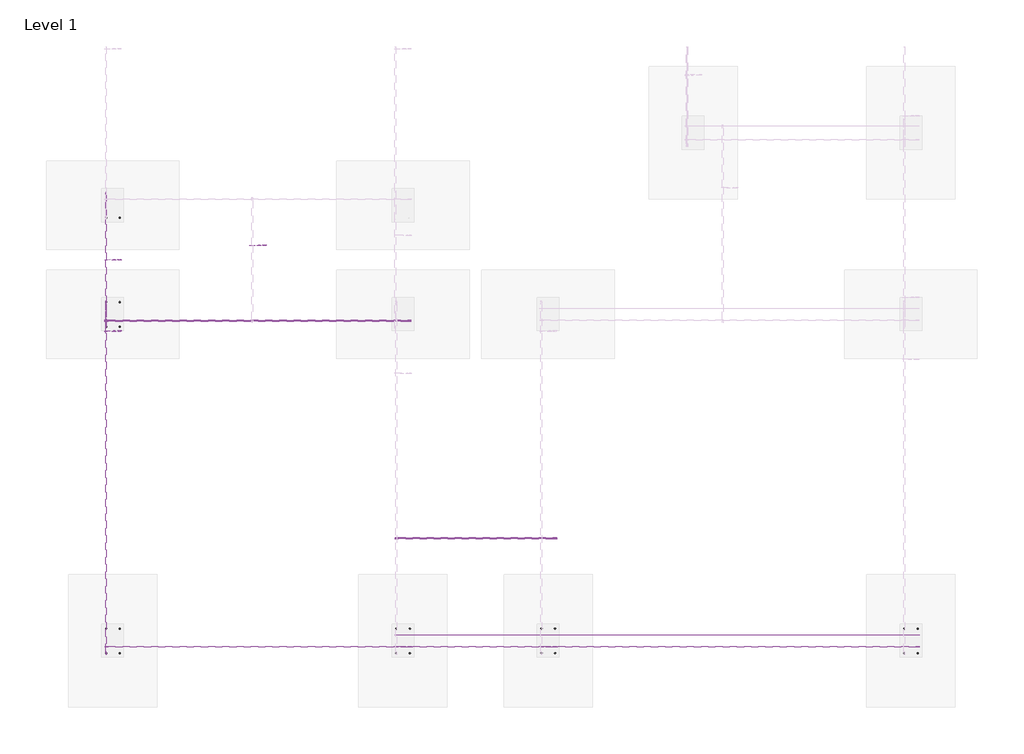
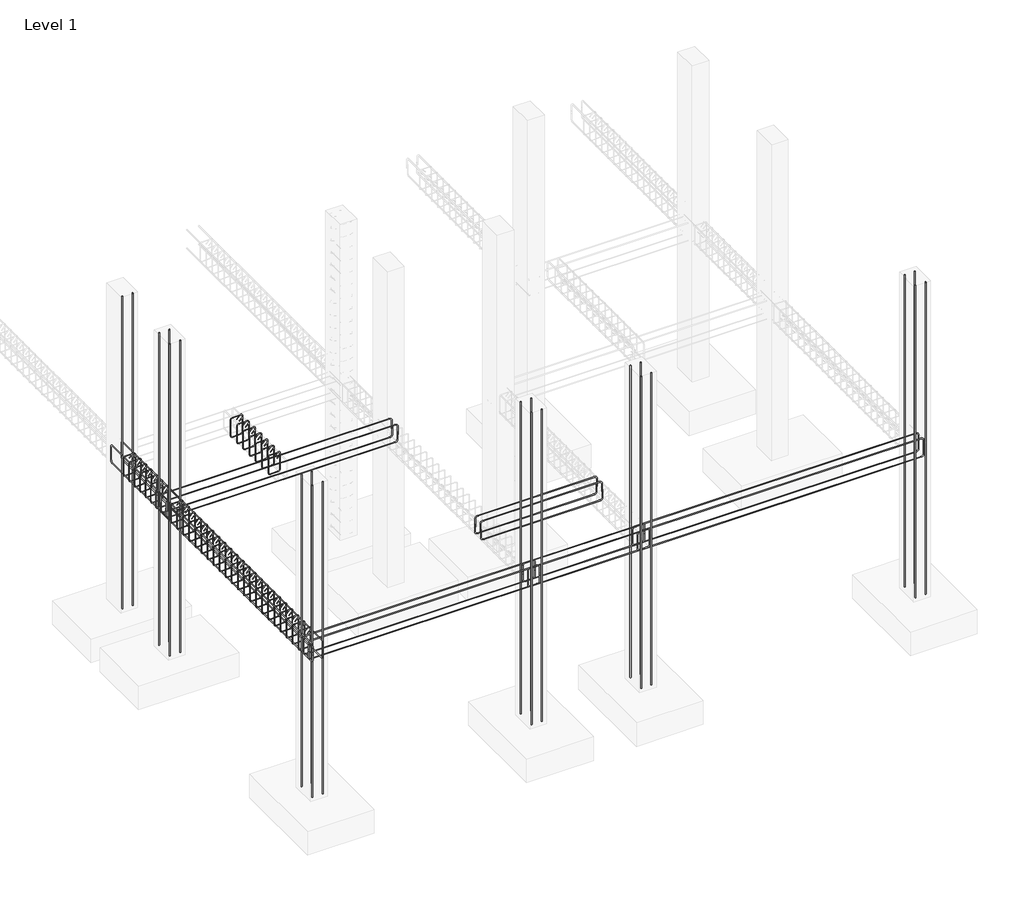
# One storey, part 2 of 5: 28 reinforcing bars.
"""IFC4 building model written with IfcOpenShell, lengths in millimetres."""

from ifc_helpers import new_model, si_unit, point, frame, origin, place, context, project, spatial, polyline, circle_curve, trimmed, segment, composite_curve, source, transform, mapped, element, save
from ifc_brep_helpers import swept_disk

model = new_model("IFC4")

# Units and contexts
model_context = context("Model", 3, world=origin())
ifc_project = project(units=[si_unit("LENGTHUNIT", "METRE", prefix="MILLI")], contexts=[model_context])

# Site, building, storey
site = spatial("IfcSite", under=ifc_project)
building = spatial("IfcBuilding", under=site)
storey = spatial("IfcBuildingStorey", under=building, Name="Level 1", Elevation=0.0)

# Reinforcing bars
placement = place(None, origin())
reinforcing_bar_shape = source(origin(), model_context, "Body", "SolidModel", [
    swept_disk(composite_curve([segment(polyline([(-4213.892587, -1952.6442969, 38.1), (-4213.892587, -1952.6442969, 6057.9)]), True, "CONTINUOUS")], self_intersect=False), 8.001),
])
element("IfcReinforcingBar", 1, at=placement, inside=storey, context=model_context, shape_type="MappedRepresentation", body=[
    mapped(reinforcing_bar_shape, transform((0.0, 0.0, 0.0), x_axis=(1.0, 0.0, 0.0), y_axis=(0.0, 1.0, 0.0), z_axis=(0.0, 0.0, 1.0))),
    mapped(reinforcing_bar_shape, transform((-186.6579018, 0.0, 0.0), x_axis=(1.0, 0.0, 0.0), y_axis=(0.0, 1.0, 0.0), z_axis=(0.0, 0.0, 1.0))),
])
reinforcing_bar_2_shape = source(origin(), model_context, "Body", "SolidModel", [
    swept_disk(composite_curve([segment(polyline([(-4213.892587, -2291.7021987, 6057.9), (-4213.892587, -2291.7021987, 38.1)]), True, "CONTINUOUS")], self_intersect=False), 8.001),
])
element("IfcReinforcingBar", 2, at=placement, inside=storey, context=model_context, shape_type="MappedRepresentation", body=[
    mapped(reinforcing_bar_2_shape, transform((0.0, 0.0, 0.0), x_axis=(1.0, 0.0, 0.0), y_axis=(0.0, 1.0, 0.0), z_axis=(0.0, 0.0, 1.0))),
    mapped(reinforcing_bar_2_shape, transform((-186.6579018, 0.0, 0.0), x_axis=(1.0, 0.0, 0.0), y_axis=(0.0, 1.0, 0.0), z_axis=(0.0, 0.0, 1.0))),
])
reinforcing_bar_3_shape = source(origin(), model_context, "Body", "SolidModel", [
    swept_disk(composite_curve([segment(polyline([(-15212.455746, 4062.3577522, 2793.8967919), (-15212.455746, 4062.3577522, 2946.2967919)]), True, "CONTINUOUS"), segment(trimmed(circle_curve(frame((-15212.455746, 4018.2887522, 2946.2967919), z_axis=(1.0, 0.0, 0.0), x_axis=(0.0, 44.06899999999996, 0.0)), 44.069), [point((-15212.455746, 4062.3577522, 2946.2967919))], [point((-15212.455746, 4018.2887522, 2990.3657919))], True, "CARTESIAN"), True, "CONTINUOUS"), segment(polyline([(-15212.455746, 4018.2887522, 2990.3657919), (-15212.455746, 2237.3647522, 2990.3657919)]), True, "CONTINUOUS"), segment(trimmed(circle_curve(frame((-15212.455746, 2237.3647522, 2946.2967919), z_axis=(1.0, 0.0, 0.0), x_axis=(0.0, 0.0, 44.069000000000415)), 44.069), [point((-15212.455746, 2237.3647522, 2990.3657919))], [point((-15212.455746, 2193.2957522, 2946.2967919))], True, "CARTESIAN"), True, "CONTINUOUS"), segment(polyline([(-15212.455746, 2193.2957522, 2946.2967919), (-15212.455746, 2193.2957522, 2793.8967919)]), True, "CONTINUOUS")], self_intersect=False), 5.969),
])
element("IfcReinforcingBar", 3, at=placement, inside=storey, context=model_context, shape_type="MappedRepresentation", body=[
    mapped(reinforcing_bar_3_shape, transform((0.0, 0.0, 0.0), x_axis=(1.0, 0.0, 0.0), y_axis=(0.0, 1.0, 0.0), z_axis=(0.0, 0.0, 1.0))),
    mapped(reinforcing_bar_3_shape, transform((-189.5315837, 0.0, 0.0), x_axis=(1.0, 0.0, 0.0), y_axis=(0.0, 1.0, 0.0), z_axis=(0.0, 0.0, 1.0))),
])
reinforcing_bar_4_shape = source(origin(), model_context, "Body", "SolidModel", [
    swept_disk(composite_curve([segment(polyline([(-15212.455746, 2193.2957522, 2844.9032081), (-15212.455746, 2193.2957522, 2692.5032081)]), True, "CONTINUOUS"), segment(trimmed(circle_curve(frame((-15212.455746, 2237.3647522, 2692.5032081), z_axis=(1.0, 0.0, 0.0), x_axis=(0.0, -44.06899999999996, 0.0)), 44.069), [point((-15212.455746, 2193.2957522, 2692.5032081))], [point((-15212.455746, 2237.3647522, 2648.4342081))], True, "CARTESIAN"), True, "CONTINUOUS"), segment(polyline([(-15212.455746, 2237.3647522, 2648.4342081), (-15212.455746, 4018.2887522, 2648.4342081)]), True, "CONTINUOUS"), segment(trimmed(circle_curve(frame((-15212.455746, 4018.2887522, 2692.5032081), z_axis=(1.0, 0.0, 0.0), x_axis=(0.0, 0.0, -44.06899999999996)), 44.069), [point((-15212.455746, 4018.2887522, 2648.4342081))], [point((-15212.455746, 4062.3577522, 2692.5032081))], True, "CARTESIAN"), True, "CONTINUOUS"), segment(polyline([(-15212.455746, 4062.3577522, 2692.5032081), (-15212.455746, 4062.3577522, 2844.9032081)]), True, "CONTINUOUS")], self_intersect=False), 5.969),
])
element("IfcReinforcingBar", 4, at=placement, inside=storey, context=model_context, shape_type="MappedRepresentation", body=[
    mapped(reinforcing_bar_4_shape, transform((0.0, 0.0, 0.0), x_axis=(1.0, 0.0, 0.0), y_axis=(0.0, 1.0, 0.0), z_axis=(0.0, 0.0, 1.0))),
    mapped(reinforcing_bar_4_shape, transform((-189.5315837, 0.0, 0.0), x_axis=(1.0, 0.0, 0.0), y_axis=(0.0, 1.0, 0.0), z_axis=(0.0, 0.0, 1.0))),
])
reinforcing_bar_5_shape = source(origin(), model_context, "Body", "SolidModel", [
    swept_disk(composite_curve([segment(polyline([(-15212.455746, 2562.3577522, 2793.8967919), (-15212.455746, 2562.3577522, 2946.2967919)]), True, "CONTINUOUS"), segment(trimmed(circle_curve(frame((-15212.455746, 2518.2887522, 2946.2967919), z_axis=(1.0, 0.0, 0.0), x_axis=(0.0, 44.06899999999996, 0.0)), 44.069), [point((-15212.455746, 2562.3577522, 2946.2967919))], [point((-15212.455746, 2518.2887522, 2990.3657919))], True, "CARTESIAN"), True, "CONTINUOUS"), segment(polyline([(-15212.455746, 2518.2887522, 2990.3657919), (-15212.455746, -2262.6352478, 2990.3657919)]), True, "CONTINUOUS"), segment(trimmed(circle_curve(frame((-15212.455746, -2262.6352478, 2946.2967919), z_axis=(1.0, 0.0, 0.0), x_axis=(0.0, 0.0, 44.069000000000415)), 44.069), [point((-15212.455746, -2262.6352478, 2990.3657919))], [point((-15212.455746, -2306.7042478, 2946.2967919))], True, "CARTESIAN"), True, "CONTINUOUS"), segment(polyline([(-15212.455746, -2306.7042478, 2946.2967919), (-15212.455746, -2306.7042478, 2793.8967919)]), True, "CONTINUOUS")], self_intersect=False), 5.969),
])
element("IfcReinforcingBar", 5, at=placement, inside=storey, context=model_context, shape_type="MappedRepresentation", body=[
    mapped(reinforcing_bar_5_shape, transform((0.0, 0.0, 0.0), x_axis=(1.0, 0.0, 0.0), y_axis=(0.0, 1.0, 0.0), z_axis=(0.0, 0.0, 1.0))),
    mapped(reinforcing_bar_5_shape, transform((-189.5315837, 0.0, 0.0), x_axis=(1.0, 0.0, 0.0), y_axis=(0.0, 1.0, 0.0), z_axis=(0.0, 0.0, 1.0))),
])
reinforcing_bar_6_shape = source(origin(), model_context, "Body", "SolidModel", [
    swept_disk(composite_curve([segment(polyline([(-15212.455746, -2306.7042478, 2844.9032081), (-15212.455746, -2306.7042478, 2692.5032081)]), True, "CONTINUOUS"), segment(trimmed(circle_curve(frame((-15212.455746, -2262.6352478, 2692.5032081), z_axis=(1.0, 0.0, 0.0), x_axis=(0.0, -44.06899999999996, 0.0)), 44.069), [point((-15212.455746, -2306.7042478, 2692.5032081))], [point((-15212.455746, -2262.6352478, 2648.4342081))], True, "CARTESIAN"), True, "CONTINUOUS"), segment(polyline([(-15212.455746, -2262.6352478, 2648.4342081), (-15212.455746, 2518.2887522, 2648.4342081)]), True, "CONTINUOUS"), segment(trimmed(circle_curve(frame((-15212.455746, 2518.2887522, 2692.5032081), z_axis=(1.0, 0.0, 0.0), x_axis=(0.0, 0.0, -44.06899999999996)), 44.069), [point((-15212.455746, 2518.2887522, 2648.4342081))], [point((-15212.455746, 2562.3577522, 2692.5032081))], True, "CARTESIAN"), True, "CONTINUOUS"), segment(polyline([(-15212.455746, 2562.3577522, 2692.5032081), (-15212.455746, 2562.3577522, 2844.9032081)]), True, "CONTINUOUS")], self_intersect=False), 5.969),
])
element("IfcReinforcingBar", 6, at=placement, inside=storey, context=model_context, shape_type="MappedRepresentation", body=[
    mapped(reinforcing_bar_6_shape, transform((0.0, 0.0, 0.0), x_axis=(1.0, 0.0, 0.0), y_axis=(0.0, 1.0, 0.0), z_axis=(0.0, 0.0, 1.0))),
    mapped(reinforcing_bar_6_shape, transform((-189.5315837, 0.0, 0.0), x_axis=(1.0, 0.0, 0.0), y_axis=(0.0, 1.0, 0.0), z_axis=(0.0, 0.0, 1.0))),
])
reinforcing_bar_7_shape = source(origin(), model_context, "Body", "SolidModel", [
    swept_disk(composite_curve([segment(polyline([(-15213.892587, 3708.2978013, 6057.9), (-15213.892587, 3708.2978013, 38.1)]), True, "CONTINUOUS")], self_intersect=False), 8.001),
])
element("IfcReinforcingBar", 7, at=placement, inside=storey, context=model_context, shape_type="MappedRepresentation", body=[
    mapped(reinforcing_bar_7_shape, transform((0.0, 0.0, 0.0), x_axis=(1.0, 0.0, 0.0), y_axis=(0.0, 1.0, 0.0), z_axis=(0.0, 0.0, 1.0))),
    mapped(reinforcing_bar_7_shape, transform((-186.6579018, 0.0, 0.0), x_axis=(1.0, 0.0, 0.0), y_axis=(0.0, 1.0, 0.0), z_axis=(0.0, 0.0, 1.0))),
])
reinforcing_bar_8_shape = source(origin(), model_context, "Body", "SolidModel", [
    swept_disk(composite_curve([segment(polyline([(-15213.892587, 2547.3557031, 38.1), (-15213.892587, 2547.3557031, 6057.9)]), True, "CONTINUOUS")], self_intersect=False), 8.001),
])
element("IfcReinforcingBar", 8, at=placement, inside=storey, context=model_context, shape_type="MappedRepresentation", body=[
    mapped(reinforcing_bar_8_shape, transform((0.0, 0.0, 0.0), x_axis=(1.0, 0.0, 0.0), y_axis=(0.0, 1.0, 0.0), z_axis=(0.0, 0.0, 1.0))),
    mapped(reinforcing_bar_8_shape, transform((-186.6579018, 0.0, 0.0), x_axis=(1.0, 0.0, 0.0), y_axis=(0.0, 1.0, 0.0), z_axis=(0.0, 0.0, 1.0))),
])
reinforcing_bar_9_shape = source(origin(), model_context, "Body", "SolidModel", [
    swept_disk(composite_curve([segment(polyline([(-15213.892587, 2208.2978013, 6057.9), (-15213.892587, 2208.2978013, 38.1)]), True, "CONTINUOUS")], self_intersect=False), 8.001),
])
element("IfcReinforcingBar", 9, at=placement, inside=storey, context=model_context, shape_type="MappedRepresentation", body=[
    mapped(reinforcing_bar_9_shape, transform((0.0, 0.0, 0.0), x_axis=(1.0, 0.0, 0.0), y_axis=(0.0, 1.0, 0.0), z_axis=(0.0, 0.0, 1.0))),
    mapped(reinforcing_bar_9_shape, transform((-186.6579018, 0.0, 0.0), x_axis=(1.0, 0.0, 0.0), y_axis=(0.0, 1.0, 0.0), z_axis=(0.0, 0.0, 1.0))),
])
reinforcing_bar_10_shape = source(origin(), model_context, "Body", "SolidModel", [
    swept_disk(composite_curve([segment(polyline([(-15213.892587, -1952.6442969, 38.1), (-15213.892587, -1952.6442969, 6057.9)]), True, "CONTINUOUS")], self_intersect=False), 8.001),
])
element("IfcReinforcingBar", 10, at=placement, inside=storey, context=model_context, shape_type="MappedRepresentation", body=[
    mapped(reinforcing_bar_10_shape, transform((0.0, 0.0, 0.0), x_axis=(1.0, 0.0, 0.0), y_axis=(0.0, 1.0, 0.0), z_axis=(0.0, 0.0, 1.0))),
    mapped(reinforcing_bar_10_shape, transform((-186.6579018, 0.0, 0.0), x_axis=(1.0, 0.0, 0.0), y_axis=(0.0, 1.0, 0.0), z_axis=(0.0, 0.0, 1.0))),
])
reinforcing_bar_11_shape = source(origin(), model_context, "Body", "SolidModel", [
    swept_disk(composite_curve([segment(polyline([(-15213.892587, -2291.7021987, 6057.9), (-15213.892587, -2291.7021987, 38.1)]), True, "CONTINUOUS")], self_intersect=False), 8.001),
])
element("IfcReinforcingBar", 11, at=placement, inside=storey, context=model_context, shape_type="MappedRepresentation", body=[
    mapped(reinforcing_bar_11_shape, transform((0.0, 0.0, 0.0), x_axis=(1.0, 0.0, 0.0), y_axis=(0.0, 1.0, 0.0), z_axis=(0.0, 0.0, 1.0))),
    mapped(reinforcing_bar_11_shape, transform((-186.6579018, 0.0, 0.0), x_axis=(1.0, 0.0, 0.0), y_axis=(0.0, 1.0, 0.0), z_axis=(0.0, 0.0, 1.0))),
])
reinforcing_bar_12_shape = source(origin(), model_context, "Body", "SolidModel", [
    swept_disk(composite_curve([segment(polyline([(-15260.3161447, 3645.2897522, 2901.0166099), (-15205.4511463, 3645.2897522, 2955.8816084)]), True, "CONTINUOUS"), segment(trimmed(circle_curve(frame((-15226.1955379, 3645.2897522, 2976.626), z_axis=(0.0, -1.0, 0.0), x_axis=(20.74439159999929, 0.0, -20.7443916000002)), 29.337), [point((-15205.4511463, 3645.2897522, 2955.8816084))], [point((-15226.1955379, 3645.2897522, 3005.963))], True, "CARTESIAN"), True, "CONTINUOUS"), segment(polyline([(-15226.1955379, 3645.2897522, 3005.963), (-15388.2475379, 3645.2897522, 3005.963)]), True, "CONTINUOUS"), segment(trimmed(circle_curve(frame((-15388.2475379, 3645.2897522, 2976.626), z_axis=(0.0, -1.0, 0.0), x_axis=(0.0, 0.0, 29.33699999999999)), 29.337), [point((-15388.2475379, 3645.2897522, 3005.963))], [point((-15417.5845379, 3645.2897522, 2976.626))], True, "CARTESIAN"), True, "CONTINUOUS"), segment(polyline([(-15417.5845379, 3645.2897522, 2976.626), (-15417.5845379, 3645.2897522, 2662.174)]), True, "CONTINUOUS"), segment(trimmed(circle_curve(frame((-15388.2661869, 3646.3356312, 2662.174), z_axis=(0.03565051078635061, -0.9993643184948482, 0.0), x_axis=(-29.318350999999893, -1.045879000000241, 0.0)), 29.337), [point((-15417.5845379, 3645.2897522, 2662.174))], [point((-15388.2661869, 3646.3356312, 2632.837))], True, "CARTESIAN"), True, "CONTINUOUS"), segment(polyline([(-15388.2661869, 3646.3356312, 2632.837), (-15226.1768889, 3652.1178731, 2632.837)]), True, "CONTINUOUS"), segment(trimmed(circle_curve(frame((-15226.1768889, 3652.1178731, 2662.174), z_axis=(0.03565051078635061, -0.9993643184948482, 0.0), x_axis=(0.0, 0.0, -29.33699999999999)), 29.337), [point((-15226.1768889, 3652.1178731, 2632.837))], [point((-15196.8585379, 3653.1637522, 2662.174))], True, "CARTESIAN"), True, "CONTINUOUS"), segment(polyline([(-15196.8585379, 3653.1637522, 2662.174), (-15196.8585379, 3653.1637522, 2976.626)]), True, "CONTINUOUS"), segment(trimmed(circle_curve(frame((-15226.1955379, 3653.1637522, 2976.626), z_axis=(0.0, -1.0, 0.0), x_axis=(29.336999999999534, 0.0, 0.0)), 29.337), [point((-15196.8585379, 3653.1637522, 2976.626))], [point((-15246.9399295, 3653.1637522, 2997.3703916))], True, "CARTESIAN"), True, "CONTINUOUS"), segment(polyline([(-15246.9399295, 3653.1637522, 2997.3703916), (-15301.804928, 3653.1637522, 2942.5053932)]), True, "CONTINUOUS")], self_intersect=False), 3.937),
])
element("IfcReinforcingBar", 12, at=placement, inside=storey, context=model_context, shape_type="MappedRepresentation", body=[
    mapped(reinforcing_bar_12_shape, transform((0.0, 0.0, 0.0), x_axis=(1.0, 0.0, 0.0), y_axis=(0.0, 1.0, 0.0), z_axis=(0.0, 0.0, 1.0))),
    mapped(reinforcing_bar_12_shape, transform((0.0, -172.4876667, 0.0), x_axis=(1.0, 0.0, 0.0), y_axis=(0.0, 1.0, 0.0), z_axis=(0.0, 0.0, 1.0))),
    mapped(reinforcing_bar_12_shape, transform((0.0, -344.9753333, 0.0), x_axis=(1.0, 0.0, 0.0), y_axis=(0.0, 1.0, 0.0), z_axis=(0.0, 0.0, 1.0))),
    mapped(reinforcing_bar_12_shape, transform((0.0, -517.463, 0.0), x_axis=(1.0, 0.0, 0.0), y_axis=(0.0, 1.0, 0.0), z_axis=(0.0, 0.0, 1.0))),
    mapped(reinforcing_bar_12_shape, transform((0.0, -689.9506667, 0.0), x_axis=(1.0, 0.0, 0.0), y_axis=(0.0, 1.0, 0.0), z_axis=(0.0, 0.0, 1.0))),
    mapped(reinforcing_bar_12_shape, transform((0.0, -862.4383333, 0.0), x_axis=(1.0, 0.0, 0.0), y_axis=(0.0, 1.0, 0.0), z_axis=(0.0, 0.0, 1.0))),
    mapped(reinforcing_bar_12_shape, transform((0.0, -1034.926, 0.0), x_axis=(1.0, 0.0, 0.0), y_axis=(0.0, 1.0, 0.0), z_axis=(0.0, 0.0, 1.0))),
])
reinforcing_bar_13_shape = source(origin(), model_context, "Body", "SolidModel", [
    swept_disk(composite_curve([segment(polyline([(-15260.3161447, 2145.2897522, 2901.0166099), (-15205.4511463, 2145.2897522, 2955.8816084)]), True, "CONTINUOUS"), segment(trimmed(circle_curve(frame((-15226.1955379, 2145.2897522, 2976.626), z_axis=(0.0, -1.0, 0.0), x_axis=(20.74439159999929, 0.0, -20.7443916000002)), 29.337), [point((-15205.4511463, 2145.2897522, 2955.8816084))], [point((-15226.1955379, 2145.2897522, 3005.963))], True, "CARTESIAN"), True, "CONTINUOUS"), segment(polyline([(-15226.1955379, 2145.2897522, 3005.963), (-15388.2475379, 2145.2897522, 3005.963)]), True, "CONTINUOUS"), segment(trimmed(circle_curve(frame((-15388.2475379, 2145.2897522, 2976.626), z_axis=(0.0, -1.0, 0.0), x_axis=(0.0, 0.0, 29.33699999999999)), 29.337), [point((-15388.2475379, 2145.2897522, 3005.963))], [point((-15417.5845379, 2145.2897522, 2976.626))], True, "CARTESIAN"), True, "CONTINUOUS"), segment(polyline([(-15417.5845379, 2145.2897522, 2976.626), (-15417.5845379, 2145.2897522, 2662.174)]), True, "CONTINUOUS"), segment(trimmed(circle_curve(frame((-15388.2661869, 2146.3356312, 2662.174), z_axis=(0.03565051078634999, -0.9993643184948483, 0.0), x_axis=(-29.318350999999893, -1.045879000000241, 0.0)), 29.337), [point((-15417.5845379, 2145.2897522, 2662.174))], [point((-15388.2661869, 2146.3356312, 2632.837))], True, "CARTESIAN"), True, "CONTINUOUS"), segment(polyline([(-15388.2661869, 2146.3356312, 2632.837), (-15226.1768889, 2152.1178731, 2632.837)]), True, "CONTINUOUS"), segment(trimmed(circle_curve(frame((-15226.1768889, 2152.1178731, 2662.174), z_axis=(0.03565051078634999, -0.9993643184948483, 0.0), x_axis=(0.0, 0.0, -29.33699999999999)), 29.337), [point((-15226.1768889, 2152.1178731, 2632.837))], [point((-15196.8585379, 2153.1637522, 2662.174))], True, "CARTESIAN"), True, "CONTINUOUS"), segment(polyline([(-15196.8585379, 2153.1637522, 2662.174), (-15196.8585379, 2153.1637522, 2976.626)]), True, "CONTINUOUS"), segment(trimmed(circle_curve(frame((-15226.1955379, 2153.1637522, 2976.626), z_axis=(0.0, -1.0, 0.0), x_axis=(29.336999999999534, 0.0, 0.0)), 29.337), [point((-15196.8585379, 2153.1637522, 2976.626))], [point((-15246.9399295, 2153.1637522, 2997.3703916))], True, "CARTESIAN"), True, "CONTINUOUS"), segment(polyline([(-15246.9399295, 2153.1637522, 2997.3703916), (-15301.804928, 2153.1637522, 2942.5053932)]), True, "CONTINUOUS")], self_intersect=False), 3.937),
])
element("IfcReinforcingBar", 13, at=placement, inside=storey, context=model_context, shape_type="MappedRepresentation", body=[
    mapped(reinforcing_bar_13_shape, transform((0.0, 0.0, 0.0), x_axis=(1.0, 0.0, 0.0), y_axis=(0.0, 1.0, 0.0), z_axis=(0.0, 0.0, 1.0))),
    mapped(reinforcing_bar_13_shape, transform((0.0, -192.1393333, 0.0), x_axis=(1.0, 0.0, 0.0), y_axis=(0.0, 1.0, 0.0), z_axis=(0.0, 0.0, 1.0))),
    mapped(reinforcing_bar_13_shape, transform((0.0, -384.2786667, 0.0), x_axis=(1.0, 0.0, 0.0), y_axis=(0.0, 1.0, 0.0), z_axis=(0.0, 0.0, 1.0))),
    mapped(reinforcing_bar_13_shape, transform((0.0, -576.418, 0.0), x_axis=(1.0, 0.0, 0.0), y_axis=(0.0, 1.0, 0.0), z_axis=(0.0, 0.0, 1.0))),
    mapped(reinforcing_bar_13_shape, transform((0.0, -768.5573333, 0.0), x_axis=(1.0, 0.0, 0.0), y_axis=(0.0, 1.0, 0.0), z_axis=(0.0, 0.0, 1.0))),
    mapped(reinforcing_bar_13_shape, transform((0.0, -960.6966667, 0.0), x_axis=(1.0, 0.0, 0.0), y_axis=(0.0, 1.0, 0.0), z_axis=(0.0, 0.0, 1.0))),
    mapped(reinforcing_bar_13_shape, transform((0.0, -1152.836, 0.0), x_axis=(1.0, 0.0, 0.0), y_axis=(0.0, 1.0, 0.0), z_axis=(0.0, 0.0, 1.0))),
    mapped(reinforcing_bar_13_shape, transform((0.0, -1344.9753333, 0.0), x_axis=(1.0, 0.0, 0.0), y_axis=(0.0, 1.0, 0.0), z_axis=(0.0, 0.0, 1.0))),
    mapped(reinforcing_bar_13_shape, transform((0.0, -1537.1146667, 0.0), x_axis=(1.0, 0.0, 0.0), y_axis=(0.0, 1.0, 0.0), z_axis=(0.0, 0.0, 1.0))),
    mapped(reinforcing_bar_13_shape, transform((0.0, -1729.254, 0.0), x_axis=(1.0, 0.0, 0.0), y_axis=(0.0, 1.0, 0.0), z_axis=(0.0, 0.0, 1.0))),
    mapped(reinforcing_bar_13_shape, transform((0.0, -1921.3933333, 0.0), x_axis=(1.0, 0.0, 0.0), y_axis=(0.0, 1.0, 0.0), z_axis=(0.0, 0.0, 1.0))),
    mapped(reinforcing_bar_13_shape, transform((0.0, -2113.5326667, 0.0), x_axis=(1.0, 0.0, 0.0), y_axis=(0.0, 1.0, 0.0), z_axis=(0.0, 0.0, 1.0))),
    mapped(reinforcing_bar_13_shape, transform((0.0, -2305.672, 0.0), x_axis=(1.0, 0.0, 0.0), y_axis=(0.0, 1.0, 0.0), z_axis=(0.0, 0.0, 1.0))),
    mapped(reinforcing_bar_13_shape, transform((0.0, -2497.8113333, 0.0), x_axis=(1.0, 0.0, 0.0), y_axis=(0.0, 1.0, 0.0), z_axis=(0.0, 0.0, 1.0))),
    mapped(reinforcing_bar_13_shape, transform((0.0, -2689.9506667, 0.0), x_axis=(1.0, 0.0, 0.0), y_axis=(0.0, 1.0, 0.0), z_axis=(0.0, 0.0, 1.0))),
    mapped(reinforcing_bar_13_shape, transform((0.0, -2882.09, 0.0), x_axis=(1.0, 0.0, 0.0), y_axis=(0.0, 1.0, 0.0), z_axis=(0.0, 0.0, 1.0))),
    mapped(reinforcing_bar_13_shape, transform((0.0, -3074.2293333, 0.0), x_axis=(1.0, 0.0, 0.0), y_axis=(0.0, 1.0, 0.0), z_axis=(0.0, 0.0, 1.0))),
    mapped(reinforcing_bar_13_shape, transform((0.0, -3266.3686667, 0.0), x_axis=(1.0, 0.0, 0.0), y_axis=(0.0, 1.0, 0.0), z_axis=(0.0, 0.0, 1.0))),
    mapped(reinforcing_bar_13_shape, transform((0.0, -3458.508, 0.0), x_axis=(1.0, 0.0, 0.0), y_axis=(0.0, 1.0, 0.0), z_axis=(0.0, 0.0, 1.0))),
    mapped(reinforcing_bar_13_shape, transform((0.0, -3650.6473333, 0.0), x_axis=(1.0, 0.0, 0.0), y_axis=(0.0, 1.0, 0.0), z_axis=(0.0, 0.0, 1.0))),
    mapped(reinforcing_bar_13_shape, transform((0.0, -3842.7866667, 0.0), x_axis=(1.0, 0.0, 0.0), y_axis=(0.0, 1.0, 0.0), z_axis=(0.0, 0.0, 1.0))),
    mapped(reinforcing_bar_13_shape, transform((0.0, -4034.926, 0.0), x_axis=(1.0, 0.0, 0.0), y_axis=(0.0, 1.0, 0.0), z_axis=(0.0, 0.0, 1.0))),
])
reinforcing_bar_14_shape = source(origin(), model_context, "Body", "SolidModel", [
    swept_disk(composite_curve([segment(polyline([(-13260.3161447, 3721.4897522, 2901.0166099), (-13205.4511463, 3721.4897522, 2955.8816084)]), True, "CONTINUOUS"), segment(trimmed(circle_curve(frame((-13226.1955379, 3721.4897522, 2976.626), z_axis=(0.0, -1.0, 0.0), x_axis=(20.74439159999929, 0.0, -20.7443916000002)), 29.337), [point((-13205.4511463, 3721.4897522, 2955.8816084))], [point((-13226.1955379, 3721.4897522, 3005.963))], True, "CARTESIAN"), True, "CONTINUOUS"), segment(polyline([(-13226.1955379, 3721.4897522, 3005.963), (-13388.2475379, 3721.4897522, 3005.963)]), True, "CONTINUOUS"), segment(trimmed(circle_curve(frame((-13388.2475379, 3721.4897522, 2976.626), z_axis=(0.0, -1.0, 0.0), x_axis=(0.0, 0.0, 29.33699999999999)), 29.337), [point((-13388.2475379, 3721.4897522, 3005.963))], [point((-13417.5845379, 3721.4897522, 2976.626))], True, "CARTESIAN"), True, "CONTINUOUS"), segment(polyline([(-13417.5845379, 3721.4897522, 2976.626), (-13417.5845379, 3721.4897522, 2662.174)]), True, "CONTINUOUS"), segment(trimmed(circle_curve(frame((-13388.2661869, 3722.5356312, 2662.174), z_axis=(0.035650510786350516, -0.9993643184948482, 0.0), x_axis=(-29.318350999999893, -1.0458789999997862, 0.0)), 29.337), [point((-13417.5845379, 3721.4897522, 2662.174))], [point((-13388.2661869, 3722.5356312, 2632.837))], True, "CARTESIAN"), True, "CONTINUOUS"), segment(polyline([(-13388.2661869, 3722.5356312, 2632.837), (-13226.1768889, 3728.3178731, 2632.837)]), True, "CONTINUOUS"), segment(trimmed(circle_curve(frame((-13226.1768889, 3728.3178731, 2662.174), z_axis=(0.035650510786350516, -0.9993643184948482, 0.0), x_axis=(0.0, 0.0, -29.33699999999999)), 29.337), [point((-13226.1768889, 3728.3178731, 2632.837))], [point((-13196.8585379, 3729.3637522, 2662.174))], True, "CARTESIAN"), True, "CONTINUOUS"), segment(polyline([(-13196.8585379, 3729.3637522, 2662.174), (-13196.8585379, 3729.3637522, 2976.626)]), True, "CONTINUOUS"), segment(trimmed(circle_curve(frame((-13226.1955379, 3729.3637522, 2976.626), z_axis=(0.0, -1.0, 0.0), x_axis=(29.336999999999534, 0.0, 0.0)), 29.337), [point((-13196.8585379, 3729.3637522, 2976.626))], [point((-13246.9399295, 3729.3637522, 2997.3703916))], True, "CARTESIAN"), True, "CONTINUOUS"), segment(polyline([(-13246.9399295, 3729.3637522, 2997.3703916), (-13301.804928, 3729.3637522, 2942.5053932)]), True, "CONTINUOUS")], self_intersect=False), 3.937),
])
element("IfcReinforcingBar", 14, at=placement, inside=storey, context=model_context, shape_type="MappedRepresentation", body=[
    mapped(reinforcing_bar_14_shape, transform((0.0, 0.0, 0.0), x_axis=(1.0, 0.0, 0.0), y_axis=(0.0, 1.0, 0.0), z_axis=(0.0, 0.0, 1.0))),
    mapped(reinforcing_bar_14_shape, transform((0.0, -197.8876667, 0.0), x_axis=(1.0, 0.0, 0.0), y_axis=(0.0, 1.0, 0.0), z_axis=(0.0, 0.0, 1.0))),
    mapped(reinforcing_bar_14_shape, transform((0.0, -395.7753333, 0.0), x_axis=(1.0, 0.0, 0.0), y_axis=(0.0, 1.0, 0.0), z_axis=(0.0, 0.0, 1.0))),
    mapped(reinforcing_bar_14_shape, transform((0.0, -593.663, 0.0), x_axis=(1.0, 0.0, 0.0), y_axis=(0.0, 1.0, 0.0), z_axis=(0.0, 0.0, 1.0))),
    mapped(reinforcing_bar_14_shape, transform((0.0, -791.5506667, 0.0), x_axis=(1.0, 0.0, 0.0), y_axis=(0.0, 1.0, 0.0), z_axis=(0.0, 0.0, 1.0))),
    mapped(reinforcing_bar_14_shape, transform((0.0, -989.4383333, 0.0), x_axis=(1.0, 0.0, 0.0), y_axis=(0.0, 1.0, 0.0), z_axis=(0.0, 0.0, 1.0))),
    mapped(reinforcing_bar_14_shape, transform((0.0, -1187.326, 0.0), x_axis=(1.0, 0.0, 0.0), y_axis=(0.0, 1.0, 0.0), z_axis=(0.0, 0.0, 1.0))),
])
reinforcing_bar_15_shape = source(origin(), model_context, "Body", "SolidModel", [
    swept_disk(composite_curve([segment(polyline([(-11198.8905379, 2283.0609603, 2793.8967919), (-11198.8905379, 2283.0609603, 2946.2967919)]), True, "CONTINUOUS"), segment(trimmed(circle_curve(frame((-11242.9595379, 2283.0609603, 2946.2967919), z_axis=(0.0, -1.0, 0.0), x_axis=(44.068999999999505, 0.0, 0.0)), 44.069), [point((-11198.8905379, 2283.0609603, 2946.2967919))], [point((-11242.9595379, 2283.0609603, 2990.3657919))], True, "CARTESIAN"), True, "CONTINUOUS"), segment(polyline([(-11242.9595379, 2283.0609603, 2990.3657919), (-15371.4835379, 2283.0609603, 2990.3657919)]), True, "CONTINUOUS"), segment(trimmed(circle_curve(frame((-15371.4835379, 2283.0609603, 2946.2967919), z_axis=(0.0, -1.0, 0.0), x_axis=(0.0, 0.0, 44.069000000000415)), 44.069), [point((-15371.4835379, 2283.0609603, 2990.3657919))], [point((-15415.5525379, 2283.0609603, 2946.2967919))], True, "CARTESIAN"), True, "CONTINUOUS"), segment(polyline([(-15415.5525379, 2283.0609603, 2946.2967919), (-15415.5525379, 2283.0609603, 2793.8967919)]), True, "CONTINUOUS")], self_intersect=False), 5.969),
])
element("IfcReinforcingBar", 15, at=placement, inside=storey, context=model_context, shape_type="MappedRepresentation", body=[
    mapped(reinforcing_bar_15_shape, transform((0.0, 0.0, 0.0), x_axis=(1.0, 0.0, 0.0), y_axis=(0.0, 1.0, 0.0), z_axis=(0.0, 0.0, 1.0))),
    mapped(reinforcing_bar_15_shape, transform((0.0, 189.5315837, 0.0), x_axis=(1.0, 0.0, 0.0), y_axis=(0.0, 1.0, 0.0), z_axis=(0.0, 0.0, 1.0))),
])
reinforcing_bar_16_shape = source(origin(), model_context, "Body", "SolidModel", [
    swept_disk(composite_curve([segment(polyline([(-15415.5525379, 2458.8527522, 2839.212), (-15415.5525379, 2458.8527522, 2686.812)]), True, "CONTINUOUS"), segment(trimmed(circle_curve(frame((-15371.4835379, 2458.8527522, 2686.812), z_axis=(0.0, -1.0, 0.0), x_axis=(-44.068999999999505, 0.0, 0.0)), 44.069), [point((-15415.5525379, 2458.8527522, 2686.812))], [point((-15371.4835379, 2458.8527522, 2642.743))], True, "CARTESIAN"), True, "CONTINUOUS"), segment(polyline([(-15371.4835379, 2458.8527522, 2642.743), (-11242.9595379, 2458.8527522, 2642.743)]), True, "CONTINUOUS"), segment(trimmed(circle_curve(frame((-11242.9595379, 2458.8527522, 2686.812), z_axis=(0.0, -1.0, 0.0), x_axis=(0.0, 0.0, -44.06899999999996)), 44.069), [point((-11242.9595379, 2458.8527522, 2642.743))], [point((-11198.8905379, 2458.8527522, 2686.812))], True, "CARTESIAN"), True, "CONTINUOUS"), segment(polyline([(-11198.8905379, 2458.8527522, 2686.812), (-11198.8905379, 2458.8527522, 2839.212)]), True, "CONTINUOUS")], self_intersect=False), 5.969),
])
element("IfcReinforcingBar", 16, at=placement, inside=storey, context=model_context, shape_type="MappedRepresentation", body=[
    mapped(reinforcing_bar_16_shape, transform((0.0, 0.0, 0.0), x_axis=(1.0, 0.0, 0.0), y_axis=(0.0, 1.0, 0.0), z_axis=(0.0, 0.0, 1.0))),
    mapped(reinforcing_bar_16_shape, transform((0.0, -162.052, 0.0), x_axis=(1.0, 0.0, 0.0), y_axis=(0.0, 1.0, 0.0), z_axis=(0.0, 0.0, 1.0))),
])
reinforcing_bar_17_shape = source(origin(), model_context, "Body", "SolidModel", [
    swept_disk(composite_curve([segment(polyline([(-11213.892587, -1952.6442969, 38.1), (-11213.892587, -1952.6442969, 6057.9)]), True, "CONTINUOUS")], self_intersect=False), 8.001),
])
element("IfcReinforcingBar", 17, at=placement, inside=storey, context=model_context, shape_type="MappedRepresentation", body=[
    mapped(reinforcing_bar_17_shape, transform((0.0, 0.0, 0.0), x_axis=(1.0, 0.0, 0.0), y_axis=(0.0, 1.0, 0.0), z_axis=(0.0, 0.0, 1.0))),
    mapped(reinforcing_bar_17_shape, transform((-186.6579018, 0.0, 0.0), x_axis=(1.0, 0.0, 0.0), y_axis=(0.0, 1.0, 0.0), z_axis=(0.0, 0.0, 1.0))),
])
reinforcing_bar_18_shape = source(origin(), model_context, "Body", "SolidModel", [
    swept_disk(composite_curve([segment(polyline([(-11213.892587, -2291.7021987, 6057.9), (-11213.892587, -2291.7021987, 38.1)]), True, "CONTINUOUS")], self_intersect=False), 8.001),
])
element("IfcReinforcingBar", 18, at=placement, inside=storey, context=model_context, shape_type="MappedRepresentation", body=[
    mapped(reinforcing_bar_18_shape, transform((0.0, 0.0, 0.0), x_axis=(1.0, 0.0, 0.0), y_axis=(0.0, 1.0, 0.0), z_axis=(0.0, 0.0, 1.0))),
    mapped(reinforcing_bar_18_shape, transform((-186.6579018, 0.0, 0.0), x_axis=(1.0, 0.0, 0.0), y_axis=(0.0, 1.0, 0.0), z_axis=(0.0, 0.0, 1.0))),
])
reinforcing_bar_19_shape = source(origin(), model_context, "Body", "SolidModel", [
    swept_disk(composite_curve([segment(polyline([(-9198.8905379, -541.1472478, 2799.588), (-9198.8905379, -541.1472478, 2951.988)]), True, "CONTINUOUS"), segment(trimmed(circle_curve(frame((-9242.9595379, -541.1472478, 2951.988), z_axis=(0.0, -1.0, 0.0), x_axis=(44.068999999999505, 0.0, 0.0)), 44.069), [point((-9198.8905379, -541.1472478, 2951.988))], [point((-9242.9595379, -541.1472478, 2996.057))], True, "CARTESIAN"), True, "CONTINUOUS"), segment(polyline([(-9242.9595379, -541.1472478, 2996.057), (-11371.4835379, -541.1472478, 2996.057)]), True, "CONTINUOUS"), segment(trimmed(circle_curve(frame((-11371.4835379, -541.1472478, 2951.988), z_axis=(0.0, -1.0, 0.0), x_axis=(0.0, 0.0, 44.06899999999996)), 44.069), [point((-11371.4835379, -541.1472478, 2996.057))], [point((-11415.5525379, -541.1472478, 2951.988))], True, "CARTESIAN"), True, "CONTINUOUS"), segment(polyline([(-11415.5525379, -541.1472478, 2951.988), (-11415.5525379, -541.1472478, 2799.588)]), True, "CONTINUOUS")], self_intersect=False), 5.969),
])
element("IfcReinforcingBar", 19, at=placement, inside=storey, context=model_context, shape_type="MappedRepresentation", body=[
    mapped(reinforcing_bar_19_shape, transform((0.0, 0.0, 0.0), x_axis=(1.0, 0.0, 0.0), y_axis=(0.0, 1.0, 0.0), z_axis=(0.0, 0.0, 1.0))),
    mapped(reinforcing_bar_19_shape, transform((0.0, -162.052, 0.0), x_axis=(1.0, 0.0, 0.0), y_axis=(0.0, 1.0, 0.0), z_axis=(0.0, 0.0, 1.0))),
])
reinforcing_bar_20_shape = source(origin(), model_context, "Body", "SolidModel", [
    swept_disk(composite_curve([segment(polyline([(-11415.5525379, -716.9390397, 2844.9032081), (-11415.5525379, -716.9390397, 2692.5032081)]), True, "CONTINUOUS"), segment(trimmed(circle_curve(frame((-11371.4835379, -716.9390397, 2692.5032081), z_axis=(0.0, -1.0, 0.0), x_axis=(-44.068999999999505, 0.0, 0.0)), 44.069), [point((-11415.5525379, -716.9390397, 2692.5032081))], [point((-11371.4835379, -716.9390397, 2648.4342081))], True, "CARTESIAN"), True, "CONTINUOUS"), segment(polyline([(-11371.4835379, -716.9390397, 2648.4342081), (-9242.9595379, -716.9390397, 2648.4342081)]), True, "CONTINUOUS"), segment(trimmed(circle_curve(frame((-9242.9595379, -716.9390397, 2692.5032081), z_axis=(0.0, -1.0, 0.0), x_axis=(0.0, 0.0, -44.06899999999996)), 44.069), [point((-9242.9595379, -716.9390397, 2648.4342081))], [point((-9198.8905379, -716.9390397, 2692.5032081))], True, "CARTESIAN"), True, "CONTINUOUS"), segment(polyline([(-9198.8905379, -716.9390397, 2692.5032081), (-9198.8905379, -716.9390397, 2844.9032081)]), True, "CONTINUOUS")], self_intersect=False), 5.969),
])
element("IfcReinforcingBar", 20, at=placement, inside=storey, context=model_context, shape_type="MappedRepresentation", body=[
    mapped(reinforcing_bar_20_shape, transform((0.0, 0.0, 0.0), x_axis=(1.0, 0.0, 0.0), y_axis=(0.0, 1.0, 0.0), z_axis=(0.0, 0.0, 1.0))),
    mapped(reinforcing_bar_20_shape, transform((0.0, 189.5315837, 0.0), x_axis=(1.0, 0.0, 0.0), y_axis=(0.0, 1.0, 0.0), z_axis=(0.0, 0.0, 1.0))),
])
reinforcing_bar_21_shape = source(origin(), model_context, "Body", "SolidModel", [
    swept_disk(composite_curve([segment(polyline([(-9213.892587, -2291.7021987, 6057.9), (-9213.892587, -2291.7021987, 38.1)]), True, "CONTINUOUS")], self_intersect=False), 8.001),
])
element("IfcReinforcingBar", 21, at=placement, inside=storey, context=model_context, shape_type="MappedRepresentation", body=[
    mapped(reinforcing_bar_21_shape, transform((0.0, 0.0, 0.0), x_axis=(1.0, 0.0, 0.0), y_axis=(0.0, 1.0, 0.0), z_axis=(0.0, 0.0, 1.0))),
    mapped(reinforcing_bar_21_shape, transform((-186.6579018, 0.0, 0.0), x_axis=(1.0, 0.0, 0.0), y_axis=(0.0, 1.0, 0.0), z_axis=(0.0, 0.0, 1.0))),
])
reinforcing_bar_22_shape = source(origin(), model_context, "Body", "SolidModel", [
    swept_disk(composite_curve([segment(polyline([(-9213.892587, -1952.6442969, 38.1), (-9213.892587, -1952.6442969, 6057.9)]), True, "CONTINUOUS")], self_intersect=False), 8.001),
])
element("IfcReinforcingBar", 22, at=placement, inside=storey, context=model_context, shape_type="MappedRepresentation", body=[
    mapped(reinforcing_bar_22_shape, transform((0.0, 0.0, 0.0), x_axis=(1.0, 0.0, 0.0), y_axis=(0.0, 1.0, 0.0), z_axis=(0.0, 0.0, 1.0))),
    mapped(reinforcing_bar_22_shape, transform((-186.6579018, 0.0, 0.0), x_axis=(1.0, 0.0, 0.0), y_axis=(0.0, 1.0, 0.0), z_axis=(0.0, 0.0, 1.0))),
])
reinforcing_bar_23_shape = source(origin(), model_context, "Body", "SolidModel", [
    swept_disk(composite_curve([segment(polyline([(-4198.8905379, -2041.1472478, 2799.588), (-4198.8905379, -2041.1472478, 2951.988)]), True, "CONTINUOUS"), segment(trimmed(circle_curve(frame((-4242.9595379, -2041.1472478, 2951.988), z_axis=(0.0, -1.0, 0.0), x_axis=(44.069000000000415, 0.0, 0.0)), 44.069), [point((-4198.8905379, -2041.1472478, 2951.988))], [point((-4242.9595379, -2041.1472478, 2996.057))], True, "CARTESIAN"), True, "CONTINUOUS"), segment(polyline([(-4242.9595379, -2041.1472478, 2996.057), (-9371.4835379, -2041.1472478, 2996.057)]), True, "CONTINUOUS"), segment(trimmed(circle_curve(frame((-9371.4835379, -2041.1472478, 2951.988), z_axis=(0.0, -1.0, 0.0), x_axis=(0.0, 0.0, 44.06899999999996)), 44.069), [point((-9371.4835379, -2041.1472478, 2996.057))], [point((-9415.5525379, -2041.1472478, 2951.988))], True, "CARTESIAN"), True, "CONTINUOUS"), segment(polyline([(-9415.5525379, -2041.1472478, 2951.988), (-9415.5525379, -2041.1472478, 2799.588)]), True, "CONTINUOUS")], self_intersect=False), 5.969),
])
element("IfcReinforcingBar", 23, at=placement, inside=storey, context=model_context, shape_type="MappedRepresentation", body=[
    mapped(reinforcing_bar_23_shape, transform((0.0, 0.0, 0.0), x_axis=(1.0, 0.0, 0.0), y_axis=(0.0, 1.0, 0.0), z_axis=(0.0, 0.0, 1.0))),
    mapped(reinforcing_bar_23_shape, transform((0.0, -162.052, 0.0), x_axis=(1.0, 0.0, 0.0), y_axis=(0.0, 1.0, 0.0), z_axis=(0.0, 0.0, 1.0))),
])
reinforcing_bar_24_shape = source(origin(), model_context, "Body", "SolidModel", [
    swept_disk(composite_curve([segment(polyline([(-9415.5525379, -2203.1992478, 2839.212), (-9415.5525379, -2203.1992478, 2686.812)]), True, "CONTINUOUS"), segment(trimmed(circle_curve(frame((-9371.4835379, -2203.1992478, 2686.812), z_axis=(0.0, -1.0, 0.0), x_axis=(-44.068999999999505, 0.0, 0.0)), 44.069), [point((-9415.5525379, -2203.1992478, 2686.812))], [point((-9371.4835379, -2203.1992478, 2642.743))], True, "CARTESIAN"), True, "CONTINUOUS"), segment(polyline([(-9371.4835379, -2203.1992478, 2642.743), (-4242.9595379, -2203.1992478, 2642.743)]), True, "CONTINUOUS"), segment(trimmed(circle_curve(frame((-4242.9595379, -2203.1992478, 2686.812), z_axis=(0.0, -1.0, 0.0), x_axis=(0.0, 0.0, -44.06899999999996)), 44.069), [point((-4242.9595379, -2203.1992478, 2642.743))], [point((-4198.8905379, -2203.1992478, 2686.812))], True, "CARTESIAN"), True, "CONTINUOUS"), segment(polyline([(-4198.8905379, -2203.1992478, 2686.812), (-4198.8905379, -2203.1992478, 2839.212)]), True, "CONTINUOUS")], self_intersect=False), 5.969),
])
element("IfcReinforcingBar", 24, at=placement, inside=storey, context=model_context, shape_type="MappedRepresentation", body=[
    mapped(reinforcing_bar_24_shape, transform((0.0, 0.0, 0.0), x_axis=(1.0, 0.0, 0.0), y_axis=(0.0, 1.0, 0.0), z_axis=(0.0, 0.0, 1.0))),
    mapped(reinforcing_bar_24_shape, transform((0.0, 162.052, 0.0), x_axis=(1.0, 0.0, 0.0), y_axis=(0.0, 1.0, 0.0), z_axis=(0.0, 0.0, 1.0))),
])
reinforcing_bar_25_shape = source(origin(), model_context, "Body", "SolidModel", [
    swept_disk(composite_curve([segment(polyline([(-9198.8905379, -2041.1472478, 2799.588), (-9198.8905379, -2041.1472478, 2951.988)]), True, "CONTINUOUS"), segment(trimmed(circle_curve(frame((-9242.9595379, -2041.1472478, 2951.988), z_axis=(0.0, -1.0, 0.0), x_axis=(44.068999999999505, 0.0, 0.0)), 44.069), [point((-9198.8905379, -2041.1472478, 2951.988))], [point((-9242.9595379, -2041.1472478, 2996.057))], True, "CARTESIAN"), True, "CONTINUOUS"), segment(polyline([(-9242.9595379, -2041.1472478, 2996.057), (-11371.4835379, -2041.1472478, 2996.057)]), True, "CONTINUOUS"), segment(trimmed(circle_curve(frame((-11371.4835379, -2041.1472478, 2951.988), z_axis=(0.0, -1.0, 0.0), x_axis=(0.0, 0.0, 44.06899999999996)), 44.069), [point((-11371.4835379, -2041.1472478, 2996.057))], [point((-11415.5525379, -2041.1472478, 2951.988))], True, "CARTESIAN"), True, "CONTINUOUS"), segment(polyline([(-11415.5525379, -2041.1472478, 2951.988), (-11415.5525379, -2041.1472478, 2799.588)]), True, "CONTINUOUS")], self_intersect=False), 5.969),
])
element("IfcReinforcingBar", 25, at=placement, inside=storey, context=model_context, shape_type="MappedRepresentation", body=[
    mapped(reinforcing_bar_25_shape, transform((0.0, 0.0, 0.0), x_axis=(1.0, 0.0, 0.0), y_axis=(0.0, 1.0, 0.0), z_axis=(0.0, 0.0, 1.0))),
    mapped(reinforcing_bar_25_shape, transform((0.0, -162.052, 0.0), x_axis=(1.0, 0.0, 0.0), y_axis=(0.0, 1.0, 0.0), z_axis=(0.0, 0.0, 1.0))),
])
reinforcing_bar_26_shape = source(origin(), model_context, "Body", "SolidModel", [
    swept_disk(composite_curve([segment(polyline([(-11415.5525379, -2203.1992478, 2839.212), (-11415.5525379, -2203.1992478, 2686.812)]), True, "CONTINUOUS"), segment(trimmed(circle_curve(frame((-11371.4835379, -2203.1992478, 2686.812), z_axis=(0.0, -1.0, 0.0), x_axis=(-44.068999999999505, 0.0, 0.0)), 44.069), [point((-11415.5525379, -2203.1992478, 2686.812))], [point((-11371.4835379, -2203.1992478, 2642.743))], True, "CARTESIAN"), True, "CONTINUOUS"), segment(polyline([(-11371.4835379, -2203.1992478, 2642.743), (-9242.9595379, -2203.1992478, 2642.743)]), True, "CONTINUOUS"), segment(trimmed(circle_curve(frame((-9242.9595379, -2203.1992478, 2686.812), z_axis=(0.0, -1.0, 0.0), x_axis=(0.0, 0.0, -44.06899999999996)), 44.069), [point((-9242.9595379, -2203.1992478, 2642.743))], [point((-9198.8905379, -2203.1992478, 2686.812))], True, "CARTESIAN"), True, "CONTINUOUS"), segment(polyline([(-9198.8905379, -2203.1992478, 2686.812), (-9198.8905379, -2203.1992478, 2839.212)]), True, "CONTINUOUS")], self_intersect=False), 5.969),
])
element("IfcReinforcingBar", 26, at=placement, inside=storey, context=model_context, shape_type="MappedRepresentation", body=[
    mapped(reinforcing_bar_26_shape, transform((0.0, 0.0, 0.0), x_axis=(1.0, 0.0, 0.0), y_axis=(0.0, 1.0, 0.0), z_axis=(0.0, 0.0, 1.0))),
    mapped(reinforcing_bar_26_shape, transform((0.0, 162.052, 0.0), x_axis=(1.0, 0.0, 0.0), y_axis=(0.0, 1.0, 0.0), z_axis=(0.0, 0.0, 1.0))),
])
reinforcing_bar_27_shape = source(origin(), model_context, "Body", "SolidModel", [
    swept_disk(composite_curve([segment(polyline([(-11198.8905379, -2041.1472478, 2799.588), (-11198.8905379, -2041.1472478, 2951.988)]), True, "CONTINUOUS"), segment(trimmed(circle_curve(frame((-11242.9595379, -2041.1472478, 2951.988), z_axis=(0.0, -1.0, 0.0), x_axis=(44.068999999999505, 0.0, 0.0)), 44.069), [point((-11198.8905379, -2041.1472478, 2951.988))], [point((-11242.9595379, -2041.1472478, 2996.057))], True, "CARTESIAN"), True, "CONTINUOUS"), segment(polyline([(-11242.9595379, -2041.1472478, 2996.057), (-15371.4835379, -2041.1472478, 2996.057)]), True, "CONTINUOUS"), segment(trimmed(circle_curve(frame((-15371.4835379, -2041.1472478, 2951.988), z_axis=(0.0, -1.0, 0.0), x_axis=(0.0, 0.0, 44.06899999999996)), 44.069), [point((-15371.4835379, -2041.1472478, 2996.057))], [point((-15415.5525379, -2041.1472478, 2951.988))], True, "CARTESIAN"), True, "CONTINUOUS"), segment(polyline([(-15415.5525379, -2041.1472478, 2951.988), (-15415.5525379, -2041.1472478, 2799.588)]), True, "CONTINUOUS")], self_intersect=False), 5.969),
])
element("IfcReinforcingBar", 27, at=placement, inside=storey, context=model_context, shape_type="MappedRepresentation", body=[
    mapped(reinforcing_bar_27_shape, transform((0.0, 0.0, 0.0), x_axis=(1.0, 0.0, 0.0), y_axis=(0.0, 1.0, 0.0), z_axis=(0.0, 0.0, 1.0))),
    mapped(reinforcing_bar_27_shape, transform((0.0, -162.052, 0.0), x_axis=(1.0, 0.0, 0.0), y_axis=(0.0, 1.0, 0.0), z_axis=(0.0, 0.0, 1.0))),
])
reinforcing_bar_28_shape = source(origin(), model_context, "Body", "SolidModel", [
    swept_disk(composite_curve([segment(polyline([(-15415.5525379, -2203.1992478, 2839.212), (-15415.5525379, -2203.1992478, 2686.812)]), True, "CONTINUOUS"), segment(trimmed(circle_curve(frame((-15371.4835379, -2203.1992478, 2686.812), z_axis=(0.0, -1.0, 0.0), x_axis=(-44.068999999999505, 0.0, 0.0)), 44.069), [point((-15415.5525379, -2203.1992478, 2686.812))], [point((-15371.4835379, -2203.1992478, 2642.743))], True, "CARTESIAN"), True, "CONTINUOUS"), segment(polyline([(-15371.4835379, -2203.1992478, 2642.743), (-11242.9595379, -2203.1992478, 2642.743)]), True, "CONTINUOUS"), segment(trimmed(circle_curve(frame((-11242.9595379, -2203.1992478, 2686.812), z_axis=(0.0, -1.0, 0.0), x_axis=(0.0, 0.0, -44.06899999999996)), 44.069), [point((-11242.9595379, -2203.1992478, 2642.743))], [point((-11198.8905379, -2203.1992478, 2686.812))], True, "CARTESIAN"), True, "CONTINUOUS"), segment(polyline([(-11198.8905379, -2203.1992478, 2686.812), (-11198.8905379, -2203.1992478, 2839.212)]), True, "CONTINUOUS")], self_intersect=False), 5.969),
])
element("IfcReinforcingBar", 28, at=placement, inside=storey, context=model_context, shape_type="MappedRepresentation", body=[
    mapped(reinforcing_bar_28_shape, transform((0.0, 0.0, 0.0), x_axis=(1.0, 0.0, 0.0), y_axis=(0.0, 1.0, 0.0), z_axis=(0.0, 0.0, 1.0))),
    mapped(reinforcing_bar_28_shape, transform((0.0, 162.052, 0.0), x_axis=(1.0, 0.0, 0.0), y_axis=(0.0, 1.0, 0.0), z_axis=(0.0, 0.0, 1.0))),
])

save(model, "model.ifc")

# Revit data of these elements
# Elements 1, 2, 3, 4, 5, 6, 7, 8, 9, 10, 11, 12, 13, 14, 15, 16, 17, 18, 19, 20, 21, 22, 23, 24, 25, 26, 27, 28 (IfcReinforcingBar)
#   Phase Created = New Construction
